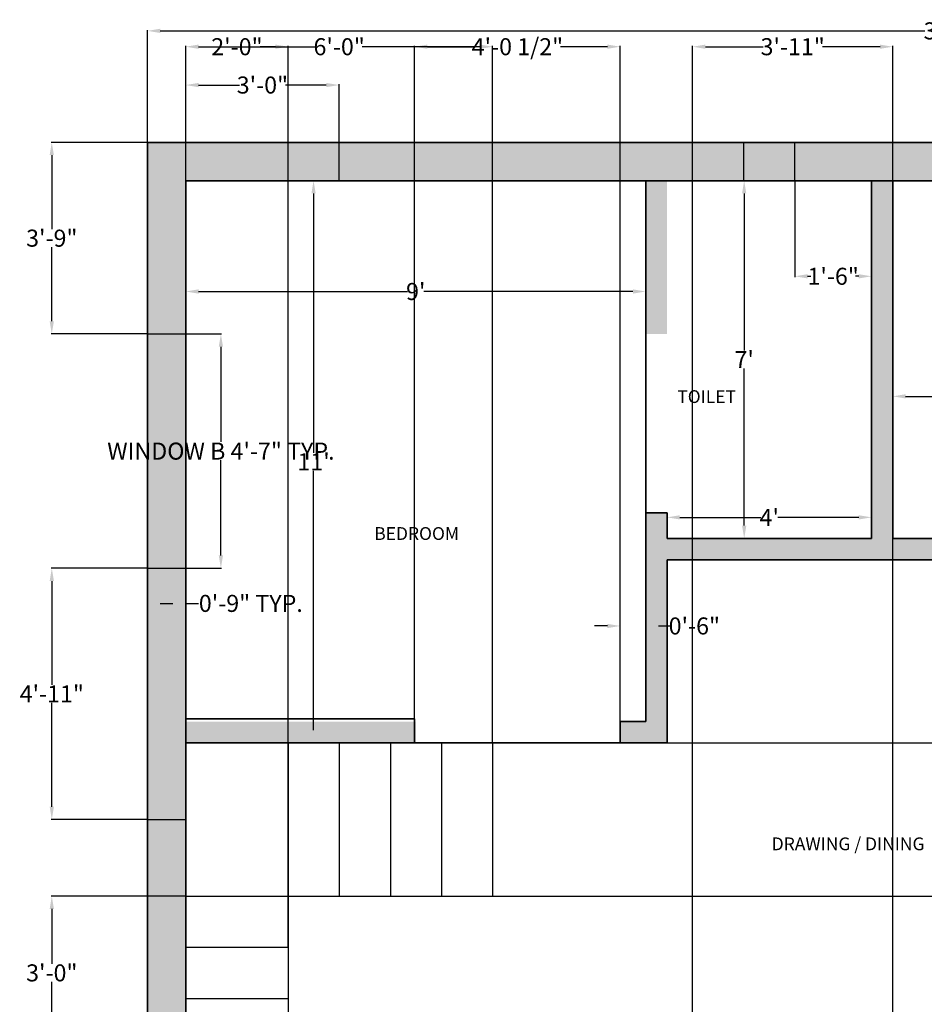
# Model space of a CAD drawing. Units: inches. Extents: x 477 to 929, y 265 to 727.
# Tile 3 of 4: x 477 to 690, y 496 to 727. Entities that reach past the tile are written whole.
import ezdxf

# ---------------------------------------------------------------- set-up
doc = ezdxf.new("R2010")
doc.units = ezdxf.units.IN
doc.header["$MEASUREMENT"] = 0
doc.layers.add('A-ANNO-DIMS', color=215, linetype='Continuous', lineweight=18, true_color=0xa953a0)
doc.layers.add('A-WALL-PATT', color=244, linetype='Continuous', lineweight=13, true_color=0x991b1e)
for name, color, linetype, lineweight in [('A-AREA-IDEN', 3, 'Continuous', 25), ('A-FLOR-STRS', 7, 'Continuous', 25), ('A-GLAZ', 4, 'Continuous', 25), ('A-GLAZ-PATT', 7, 'Continuous', 13), ('A-WALL', 7, 'Continuous', 35)]:
    doc.layers.add(name, color=color, linetype=linetype, lineweight=lineweight)
doc.styles.get("Standard").update_dxf_attribs({"font": 'arial.ttf'})
doc.dimstyles.get("Standard").update_dxf_attribs({"dimtxt": 4, "dimasz": 3, "dimexe": 0.18, "dimexo": 0.0625, "dimgap": 0.09, "dimtad": 0, "dimtih": 1, "dimtoh": 1, "dimdec": 0, "dimzin": 0, "dimdsep": 46, "dimlunit": 3, "dimtxsty": 'Standard', "dimcen": 0, "dimadec": 0, "dimazin": 0, "dimtfac": 1, "dimtdec": 0, "dimtofl": 0, "dimtmove": 0, "dimatfit": 3, "dimfxl": 1, "dimtolj": 1, "dimtzin": 0, "dimarcsym": 1})

# ---------------------------------------------------------------- blocks, each defined once
blk = doc.blocks.new('*D11')
at = {"layer": 'A-ANNO-DIMS', "color": 0, "lineweight": -2, "transparency": 16777216}
for p, q in [((682.33, 605.27), (682.33, 638.75)), ((685.33, 638.57), (704.32, 638.57)), ((727.33, 638.57), (708.34, 638.57)), ((730.33, 605.27), (730.33, 638.75))]:
    blk.add_line(p, q, dxfattribs=at)
at = {"layer": 'A-ANNO-DIMS', "color": 0, "transparency": 16777216}
for points in [[(685.33, 639.07), (685.33, 638.07), (682.33, 638.57)], [(727.33, 639.07), (727.33, 638.07), (730.33, 638.57)]]:
    blk.add_solid(points, dxfattribs=at)
at = {"layer": 'Defpoints', "color": 0, "transparency": 16777216}
for p in [(730.33, 638.57), (682.33, 605.21), (730.33, 605.21)]:
    blk.add_point(p, dxfattribs=at)
at = {"layer": 'A-ANNO-DIMS', "color": 0, "transparency": 16777216, "insert": (706.33, 638.57), "char_height": 4, "attachment_point": 5}
blk.add_mtext("\\A1;4'", dxfattribs=at)
blk = doc.blocks.new('*D13')
at = {"layer": 'A-ANNO-DIMS', "color": 0, "lineweight": -2, "transparency": 16777216}
for p, q in [((629.33, 611.14), (629.33, 609.98)), ((677.33, 611.14), (677.33, 609.98)), ((632.33, 610.16), (651.32, 610.16)), ((674.33, 610.16), (655.34, 610.16))]:
    blk.add_line(p, q, dxfattribs=at)
at = {"layer": 'A-ANNO-DIMS', "color": 0, "transparency": 16777216}
for points in [[(632.33, 610.66), (632.33, 609.66), (629.33, 610.16)], [(674.33, 610.66), (674.33, 609.66), (677.33, 610.16)]]:
    blk.add_solid(points, dxfattribs=at)
at = {"layer": 'Defpoints', "color": 0, "transparency": 16777216}
for p in [(629.33, 611.21), (677.33, 611.21), (677.33, 610.16)]:
    blk.add_point(p, dxfattribs=at)
at = {"layer": 'A-ANNO-DIMS', "color": 0, "transparency": 16777216, "insert": (653.33, 610.16), "char_height": 4, "attachment_point": 5}
blk.add_mtext("\\A1;4'", dxfattribs=at)
blk = doc.blocks.new('*D14')
at = {"layer": 'A-ANNO-DIMS', "color": 0, "lineweight": -2, "transparency": 16777216}
for p, q in [((653.07, 689.21), (647.26, 689.21)), ((647.44, 686.21), (647.44, 649.3)), ((647.44, 608.21), (647.44, 645.12)), ((653.27, 605.21), (647.26, 605.21))]:
    blk.add_line(p, q, dxfattribs=at)
at = {"layer": 'A-ANNO-DIMS', "color": 0, "transparency": 16777216}
for points in [[(646.94, 686.21), (647.94, 686.21), (647.44, 689.21)], [(646.94, 608.21), (647.94, 608.21), (647.44, 605.21)]]:
    blk.add_solid(points, dxfattribs=at)
at = {"layer": 'Defpoints', "color": 0, "transparency": 16777216}
for p in [(653.13, 689.21), (647.44, 605.21), (653.33, 605.21)]:
    blk.add_point(p, dxfattribs=at)
at = {"layer": 'A-ANNO-DIMS', "color": 0, "transparency": 16777216, "insert": (647.44, 647.21), "char_height": 4, "attachment_point": 5}
blk.add_mtext("\\A1;7'", dxfattribs=at)
blk = doc.blocks.new('*D15')
at = {"layer": 'A-ANNO-DIMS', "color": 0, "lineweight": -2, "transparency": 16777216}
for p, q in [((570.81, 689.21), (546.16, 689.21)), ((546.34, 686.21), (546.34, 625.3)), ((546.34, 560.21), (546.34, 621.11)), ((572.77, 557.21), (546.16, 557.21))]:
    blk.add_line(p, q, dxfattribs=at)
at = {"layer": 'A-ANNO-DIMS', "color": 0, "transparency": 16777216}
for points in [[(545.84, 686.21), (546.84, 686.21), (546.34, 689.21)], [(545.84, 560.21), (546.84, 560.21), (546.34, 557.21)]]:
    blk.add_solid(points, dxfattribs=at)
at = {"layer": 'Defpoints', "color": 0, "transparency": 16777216}
for p in [(570.87, 689.21), (546.34, 557.21), (572.83, 557.21)]:
    blk.add_point(p, dxfattribs=at)
at = {"layer": 'A-ANNO-DIMS', "color": 0, "transparency": 16777216, "insert": (546.34, 623.21), "char_height": 4, "attachment_point": 5}
blk.add_mtext("\\A1;11'", dxfattribs=at)
blk = doc.blocks.new('*D16')
at = {"layer": 'A-ANNO-DIMS', "color": 0, "lineweight": -2, "transparency": 16777216}
for p, q in [((516.33, 661.56), (516.33, 663.37)), ((519.33, 663.19), (568.4, 663.19)), ((621.33, 663.19), (572.26, 663.19)), ((624.33, 661.56), (624.33, 663.37))]:
    blk.add_line(p, q, dxfattribs=at)
at = {"layer": 'A-ANNO-DIMS', "color": 0, "transparency": 16777216}
for points in [[(519.33, 663.69), (519.33, 662.69), (516.33, 663.19)], [(621.33, 663.69), (621.33, 662.69), (624.33, 663.19)]]:
    blk.add_solid(points, dxfattribs=at)
at = {"layer": 'Defpoints', "color": 0, "transparency": 16777216}
for p in [(516.33, 661.5), (624.33, 663.19), (624.33, 661.5)]:
    blk.add_point(p, dxfattribs=at)
at = {"layer": 'A-ANNO-DIMS', "color": 0, "transparency": 16777216, "insert": (570.33, 663.19), "char_height": 4, "attachment_point": 5}
blk.add_mtext("\\A1;9'", dxfattribs=at)
blk = doc.blocks.new('*D18')
at = {"layer": 'A-ANNO-DIMS', "color": 0, "lineweight": -2, "transparency": 16777216}
for p, q in [((507.33, 698.27), (507.33, 724.56)), ((510.33, 724.38), (689.88, 724.38)), ((876.4, 724.38), (696.85, 724.38)), ((879.4, 698.27), (879.4, 724.56))]:
    blk.add_line(p, q, dxfattribs=at)
at = {"layer": 'A-ANNO-DIMS', "color": 0, "transparency": 16777216}
for points in [[(510.33, 724.88), (510.33, 723.88), (507.33, 724.38)], [(876.4, 724.88), (876.4, 723.88), (879.4, 724.38)]]:
    blk.add_solid(points, dxfattribs=at)
at = {"layer": 'Defpoints', "color": 0, "transparency": 16777216}
for p in [(879.4, 724.38), (507.33, 698.21), (879.4, 698.21)]:
    blk.add_point(p, dxfattribs=at)
at = {"layer": 'A-ANNO-DIMS', "color": 0, "transparency": 16777216, "insert": (693.36, 724.38), "char_height": 4, "attachment_point": 5}
blk.add_mtext("\\A1;31'", dxfattribs=at)
blk = doc.blocks.new('WIN-JAMBS-36IN')
for p, q in [((9, 36), (0, 36)), ((9, 0), (0, 0))]:
    blk.add_line(p, q)
blk = doc.blocks.new('WIN-JAMBS-55IN')
for p, q in [((0, 55), (9, 55)), ((0, 0), (9, 0))]:
    blk.add_line(p, q)
blk = doc.blocks.new('WIN-JAMBS-12IN')
for p, q in [((0, 0), (0, 9)), ((12, 0), (12, 9))]:
    blk.add_line(p, q)
blk = doc.blocks.new('*D25')
at = {"layer": 'A-ANNO-DIMS', "color": 0, "lineweight": -2, "transparency": 16777216}
for p, q in [((516.4, 653.21), (524.76, 653.21)), ((524.58, 650.21), (524.58, 627.86)), ((524.58, 601.21), (524.58, 623.55)), ((516.4, 598.21), (524.76, 598.21))]:
    blk.add_line(p, q, dxfattribs=at)
at = {"layer": 'A-ANNO-DIMS', "color": 0, "transparency": 16777216}
for points in [[(524.08, 650.21), (525.08, 650.21), (524.58, 653.21)], [(524.08, 601.21), (525.08, 601.21), (524.58, 598.21)]]:
    blk.add_solid(points, dxfattribs=at)
at = {"layer": 'Defpoints', "color": 0, "transparency": 16777216}
for p in [(516.33, 653.21), (524.58, 653.21), (516.33, 598.21)]:
    blk.add_point(p, dxfattribs=at)
at = {"layer": 'A-ANNO-DIMS', "color": 0, "transparency": 16777216, "insert": (524.58, 625.71), "char_height": 4, "attachment_point": 5}
blk.add_mtext('\\A1;WINDOW B 4\'-7" TYP.', dxfattribs=at)
blk = doc.blocks.new('*D26')
at = {"layer": 'A-ANNO-DIMS', "color": 0, "lineweight": -2, "transparency": 16777216}
for p, q in [((507.33, 598.14), (507.33, 589.78)), ((516.33, 598.14), (516.33, 589.78)), ((510.33, 589.96), (513.33, 589.96)), ((516.33, 589.96), (519.33, 589.96))]:
    blk.add_line(p, q, dxfattribs=at)
at = {"layer": 'A-ANNO-DIMS', "color": 0, "transparency": 16777216}
for points in [[(510.33, 590.46), (510.33, 589.46), (507.33, 589.96)], [(513.33, 590.46), (513.33, 589.46), (516.33, 589.96)]]:
    blk.add_solid(points, dxfattribs=at)
at = {"layer": 'Defpoints', "color": 0, "transparency": 16777216}
for p in [(507.33, 598.21), (516.33, 598.21), (516.33, 589.96)]:
    blk.add_point(p, dxfattribs=at)
at = {"layer": 'A-ANNO-DIMS', "color": 0, "transparency": 16777216, "insert": (531.61, 589.96), "char_height": 4, "attachment_point": 5}
blk.add_mtext('\\A1;0\'-9" TYP.', dxfattribs=at)
blk = doc.blocks.new('*D30')
at = {"layer": 'A-ANNO-DIMS', "color": 0, "lineweight": -2, "transparency": 16777216}
for p, q in [((588.43, 557.21), (901.96, 557.21)), ((901.78, 554.21), (901.78, 541.34)), ((901.78, 524.21), (901.78, 537.07)), ((588.43, 521.21), (901.96, 521.21))]:
    blk.add_line(p, q, dxfattribs=at)
at = {"layer": 'A-ANNO-DIMS', "color": 0, "transparency": 16777216}
for points in [[(901.28, 554.21), (902.28, 554.21), (901.78, 557.21)], [(901.28, 524.21), (902.28, 524.21), (901.78, 521.21)]]:
    blk.add_solid(points, dxfattribs=at)
at = {"layer": 'Defpoints', "color": 0, "transparency": 16777216}
for p in [(588.37, 557.21), (901.78, 557.21), (588.37, 521.21)]:
    blk.add_point(p, dxfattribs=at)
at = {"layer": 'A-ANNO-DIMS', "color": 0, "transparency": 16777216, "insert": (901.78, 539.21), "char_height": 4, "attachment_point": 5}
blk.add_mtext('\\A1;3\'-0"', dxfattribs=at)
blk = doc.blocks.new('*D32')
at = {"layer": 'A-ANNO-DIMS', "color": 0, "lineweight": -2, "transparency": 16777216}
for p, q in [((516.33, 509.27), (516.33, 720.84)), ((519.33, 720.66), (522.91, 720.66)), ((537.37, 720.66), (533.79, 720.66)), ((540.37, 509.27), (540.37, 720.84))]:
    blk.add_line(p, q, dxfattribs=at)
at = {"layer": 'A-ANNO-DIMS', "color": 0, "transparency": 16777216}
for points in [[(519.33, 721.16), (519.33, 720.16), (516.33, 720.66)], [(537.37, 721.16), (537.37, 720.16), (540.37, 720.66)]]:
    blk.add_solid(points, dxfattribs=at)
at = {"layer": 'Defpoints', "color": 0, "transparency": 16777216}
for p in [(540.37, 720.66), (516.33, 509.21), (540.37, 509.21)]:
    blk.add_point(p, dxfattribs=at)
at = {"layer": 'A-ANNO-DIMS', "color": 0, "transparency": 16777216, "insert": (528.35, 720.66), "char_height": 4, "attachment_point": 5}
blk.add_mtext('\\A1;2\'-0"', dxfattribs=at)
blk = doc.blocks.new('*D33')
at = {"layer": 'A-ANNO-DIMS', "color": 0, "lineweight": -2, "transparency": 16777216}
for p, q in [((516.33, 557.27), (516.33, 720.84)), ((519.33, 720.66), (546.93, 720.66)), ((585.37, 720.66), (557.77, 720.66)), ((588.37, 557.27), (588.37, 720.84))]:
    blk.add_line(p, q, dxfattribs=at)
at = {"layer": 'A-ANNO-DIMS', "color": 0, "transparency": 16777216}
for points in [[(519.33, 721.16), (519.33, 720.16), (516.33, 720.66)], [(585.37, 721.16), (585.37, 720.16), (588.37, 720.66)]]:
    blk.add_solid(points, dxfattribs=at)
at = {"layer": 'Defpoints', "color": 0, "transparency": 16777216}
for p in [(588.37, 720.66), (516.33, 557.21), (588.37, 557.21)]:
    blk.add_point(p, dxfattribs=at)
at = {"layer": 'A-ANNO-DIMS', "color": 0, "transparency": 16777216, "insert": (552.35, 720.66), "char_height": 4, "attachment_point": 5}
blk.add_mtext('\\A1;6\'-0"', dxfattribs=at)
blk = doc.blocks.new('*D35')
at = {"layer": 'A-ANNO-DIMS', "color": 0, "lineweight": -2, "transparency": 16777216}
for p, q in [((516.27, 521.21), (484.7, 521.21)), ((484.88, 518.21), (484.88, 505.34)), ((484.88, 488.21), (484.88, 501.07)), ((516.27, 485.21), (484.7, 485.21))]:
    blk.add_line(p, q, dxfattribs=at)
at = {"layer": 'A-ANNO-DIMS', "color": 0, "transparency": 16777216}
for points in [[(484.38, 518.21), (485.38, 518.21), (484.88, 521.21)], [(484.38, 488.21), (485.38, 488.21), (484.88, 485.21)]]:
    blk.add_solid(points, dxfattribs=at)
at = {"layer": 'Defpoints', "color": 0, "transparency": 16777216}
for p in [(484.88, 521.21), (516.33, 521.21), (516.33, 485.21)]:
    blk.add_point(p, dxfattribs=at)
at = {"layer": 'A-ANNO-DIMS', "color": 0, "transparency": 16777216, "insert": (484.88, 503.21), "char_height": 4, "attachment_point": 5}
blk.add_mtext('\\A1;3\'-0"', dxfattribs=at)
blk = doc.blocks.new('*D40')
at = {"layer": 'A-ANNO-DIMS', "color": 0, "lineweight": -2, "transparency": 16777216}
for p, q in [((516.33, 689.27), (516.33, 711.84)), ((519.33, 711.66), (528.93, 711.66)), ((549.33, 711.66), (539.74, 711.66)), ((552.33, 689.27), (552.33, 711.84))]:
    blk.add_line(p, q, dxfattribs=at)
at = {"layer": 'A-ANNO-DIMS', "color": 0, "transparency": 16777216}
for points in [[(519.33, 712.16), (519.33, 711.16), (516.33, 711.66)], [(549.33, 712.16), (549.33, 711.16), (552.33, 711.66)]]:
    blk.add_solid(points, dxfattribs=at)
at = {"layer": 'Defpoints', "color": 0, "transparency": 16777216}
for p in [(552.33, 711.66), (516.33, 689.21), (552.33, 689.21)]:
    blk.add_point(p, dxfattribs=at)
at = {"layer": 'A-ANNO-DIMS', "color": 0, "transparency": 16777216, "insert": (534.33, 711.66), "char_height": 4, "attachment_point": 5}
blk.add_mtext('\\A1;3\'-0"', dxfattribs=at)
blk = doc.blocks.new('*D41')
at = {"layer": 'A-ANNO-DIMS', "color": 0, "lineweight": -2, "transparency": 16777216}
for p, q in [((659.33, 689.14), (659.33, 666.58)), ((677.33, 689.14), (677.33, 666.58)), ((662.33, 666.76), (663.12, 666.76)), ((674.33, 666.76), (673.55, 666.76))]:
    blk.add_line(p, q, dxfattribs=at)
at = {"layer": 'A-ANNO-DIMS', "color": 0, "transparency": 16777216}
for points in [[(662.33, 667.26), (662.33, 666.26), (659.33, 666.76)], [(674.33, 667.26), (674.33, 666.26), (677.33, 666.76)]]:
    blk.add_solid(points, dxfattribs=at)
at = {"layer": 'Defpoints', "color": 0, "transparency": 16777216}
for p in [(659.33, 689.21), (677.33, 689.21), (659.33, 666.76)]:
    blk.add_point(p, dxfattribs=at)
at = {"layer": 'A-ANNO-DIMS', "color": 0, "transparency": 16777216, "insert": (668.33, 666.76), "char_height": 4, "attachment_point": 5}
blk.add_mtext('\\A1;1\'-6"', dxfattribs=at)
blk = doc.blocks.new('*D45')
at = {"layer": 'A-ANNO-DIMS', "color": 0, "lineweight": -2, "transparency": 16777216}
for p, q in [((507.27, 698.21), (484.7, 698.21)), ((484.88, 695.21), (484.88, 677.84)), ((484.88, 656.21), (484.88, 673.57)), ((507.27, 653.21), (484.7, 653.21))]:
    blk.add_line(p, q, dxfattribs=at)
at = {"layer": 'A-ANNO-DIMS', "color": 0, "transparency": 16777216}
for points in [[(484.38, 695.21), (485.38, 695.21), (484.88, 698.21)], [(484.38, 656.21), (485.38, 656.21), (484.88, 653.21)]]:
    blk.add_solid(points, dxfattribs=at)
at = {"layer": 'Defpoints', "color": 0, "transparency": 16777216}
for p in [(484.88, 698.21), (507.33, 698.21), (507.33, 653.21)]:
    blk.add_point(p, dxfattribs=at)
at = {"layer": 'A-ANNO-DIMS', "color": 0, "transparency": 16777216, "insert": (484.88, 675.71), "char_height": 4, "attachment_point": 5}
blk.add_mtext('\\A1;3\'-9"', dxfattribs=at)
blk = doc.blocks.new('*D46')
at = {"layer": 'A-ANNO-DIMS', "color": 0, "lineweight": -2, "transparency": 16777216}
for p, q in [((507.27, 598.21), (484.7, 598.21)), ((484.88, 595.21), (484.88, 570.8)), ((484.88, 542.21), (484.88, 566.61)), ((507.27, 539.21), (484.7, 539.21))]:
    blk.add_line(p, q, dxfattribs=at)
at = {"layer": 'A-ANNO-DIMS', "color": 0, "transparency": 16777216}
for points in [[(484.38, 595.21), (485.38, 595.21), (484.88, 598.21)], [(484.38, 542.21), (485.38, 542.21), (484.88, 539.21)]]:
    blk.add_solid(points, dxfattribs=at)
at = {"layer": 'Defpoints', "color": 0, "transparency": 16777216}
for p in [(484.88, 598.21), (507.33, 598.21), (507.33, 539.21)]:
    blk.add_point(p, dxfattribs=at)
at = {"layer": 'A-ANNO-DIMS', "color": 0, "transparency": 16777216, "insert": (484.88, 568.71), "char_height": 4, "attachment_point": 5}
blk.add_mtext('\\A1;4\'-11"', dxfattribs=at)
blk = doc.blocks.new('*D57')
at = {"layer": 'A-ANNO-DIMS', "color": 0, "lineweight": -2, "transparency": 16777216}
for p, q in [((635.33, 400.27), (635.33, 720.84)), ((638.33, 720.66), (651.87, 720.66)), ((679.33, 720.66), (665.79, 720.66)), ((682.33, 400.27), (682.33, 720.84))]:
    blk.add_line(p, q, dxfattribs=at)
at = {"layer": 'A-ANNO-DIMS', "color": 0, "transparency": 16777216}
for points in [[(638.33, 721.16), (638.33, 720.16), (635.33, 720.66)], [(679.33, 721.16), (679.33, 720.16), (682.33, 720.66)]]:
    blk.add_solid(points, dxfattribs=at)
at = {"layer": 'Defpoints', "color": 0, "transparency": 16777216}
for p in [(682.33, 720.66), (635.33, 400.21), (682.33, 400.21)]:
    blk.add_point(p, dxfattribs=at)
at = {"layer": 'A-ANNO-DIMS', "color": 0, "transparency": 16777216, "insert": (658.83, 720.66), "char_height": 4, "attachment_point": 5}
blk.add_mtext('\\A1;3\'-11"', dxfattribs=at)
blk = doc.blocks.new('*D61')
at = {"layer": 'A-ANNO-DIMS', "color": 0, "lineweight": -2, "transparency": 16777216}
for p, q in [((570.07, 562.88), (570.07, 720.84)), ((573.07, 720.66), (584.05, 720.66)), ((615.33, 720.66), (604.35, 720.66)), ((618.33, 562.27), (618.33, 720.84))]:
    blk.add_line(p, q, dxfattribs=at)
at = {"layer": 'A-ANNO-DIMS', "color": 0, "transparency": 16777216}
for points in [[(573.07, 721.16), (573.07, 720.16), (570.07, 720.66)], [(615.33, 721.16), (615.33, 720.16), (618.33, 720.66)]]:
    blk.add_solid(points, dxfattribs=at)
at = {"layer": 'Defpoints', "color": 0, "transparency": 16777216}
for p in [(570.07, 720.66), (570.07, 562.82), (618.33, 562.21)]:
    blk.add_point(p, dxfattribs=at)
at = {"layer": 'A-ANNO-DIMS', "color": 0, "transparency": 16777216, "insert": (594.2, 720.66), "char_height": 4, "attachment_point": 5}
blk.add_mtext('\\A1;4\'-0 1/2"', dxfattribs=at)
blk = doc.blocks.new('*D68')
at = {"layer": 'A-ANNO-DIMS', "color": 0, "lineweight": -2, "transparency": 16777216}
for p, q in [((615.33, 584.66), (612.33, 584.66)), ((618.33, 562.27), (618.33, 584.84)), ((624.33, 562.27), (624.33, 584.84)), ((627.33, 584.66), (630.33, 584.66))]:
    blk.add_line(p, q, dxfattribs=at)
at = {"layer": 'A-ANNO-DIMS', "color": 0, "transparency": 16777216}
for points in [[(615.33, 585.16), (615.33, 584.16), (618.33, 584.66)], [(627.33, 585.16), (627.33, 584.16), (624.33, 584.66)]]:
    blk.add_solid(points, dxfattribs=at)
at = {"layer": 'Defpoints', "color": 0, "transparency": 16777216}
for p in [(624.33, 584.66), (618.33, 562.21), (624.33, 562.21)]:
    blk.add_point(p, dxfattribs=at)
at = {"layer": 'A-ANNO-DIMS', "color": 0, "transparency": 16777216, "insert": (635.74, 584.66), "char_height": 4, "attachment_point": 5}
blk.add_mtext('\\A1;0\'-6"', dxfattribs=at)

msp = doc.modelspace()

# ---------------------------------------------------------------- hatches: boundary and pattern name
at = {"layer": 'A-GLAZ-PATT'}
h = msp.add_hatch(color=256, dxfattribs=at)
h.dxf.hatch_style = 1
h.paths.add_polyline_path([(588.33, 698.21), (552.33, 698.21), (552.33, 689.21), (588.33, 689.21)])
h.paths.add_polyline_path([(659.33, 698.21), (647.33, 698.21), (647.33, 689.21), (659.33, 689.21)])
h.paths.add_polyline_path([(712.33, 698.21), (700.33, 698.21), (700.33, 689.21), (712.33, 689.21)])
h.paths.add_polyline_path([(834.33, 698.21), (771.33, 698.21), (771.33, 689.21), (834.33, 689.21)])
h.paths.add_polyline_path([(879.33, 653.21), (870.33, 653.21), (870.33, 598.21), (879.33, 598.21)])
h.paths.add_polyline_path([(879.33, 521.21), (870.33, 521.21), (870.33, 484.21), (879.33, 484.21)])
h.paths.add_polyline_path([(879.33, 407.21), (870.33, 407.21), (870.33, 371.21), (879.33, 371.21)])
h.paths.add_polyline_path([(834.33, 335.21), (766.33, 335.21), (766.33, 326.21), (834.33, 326.21)])
h.paths.add_polyline_path([(588.33, 335.21), (552.33, 335.21), (552.33, 326.21), (588.33, 326.21)])
h.paths.add_polyline_path([(516.33, 430.21), (507.33, 430.21), (507.33, 371.21), (516.33, 371.21)])
h.paths.add_polyline_path([(516.33, 539.21), (507.33, 539.21), (507.33, 466.21), (516.33, 466.21)])
h.paths.add_polyline_path([(516.33, 653.21), (507.33, 653.21), (507.33, 598.21), (516.33, 598.21)])
at = {"layer": 'A-WALL-PATT'}
h = msp.add_hatch(color=256, dxfattribs=at)
h.dxf.hatch_style = 1
h.paths.add_polyline_path([(516.33, 598.21), (507.33, 598.21), (507.33, 539.21), (516.33, 539.21), (516.33, 557.21), (570.33, 557.21), (570.33, 562.21), (516.33, 562.21)])
h.paths.add_polyline_path([(552.33, 698.21), (507.33, 698.21), (507.33, 653.21), (516.33, 653.21), (516.33, 689.21), (552.33, 689.21)])
h.paths.add_polyline_path([(647.33, 698.21), (588.33, 698.21), (588.33, 689.21), (647.33, 689.21)])
h.paths.add_polyline_path([(700.33, 698.21), (659.33, 698.21), (659.33, 689.21), (700.33, 689.21)])
h.paths.add_polyline_path([(771.33, 698.21), (712.33, 698.21), (712.33, 689.21), (771.33, 689.21)])
h.paths.add_polyline_path([(879.33, 698.21), (834.33, 698.21), (834.33, 689.21), (870.33, 689.21), (870.33, 653.21), (879.33, 653.21)])
h.paths.add_polyline_path([(879.33, 598.21), (870.33, 598.21), (870.33, 562.21), (735.33, 562.21), (735.33, 568.21), (730.33, 568.21), (730.33, 557.21), (793.33, 557.21), (793.33, 551.21), (798.33, 551.21), (798.33, 557.21), (870.33, 557.21), (870.33, 521.21), (879.33, 521.21)])
h.paths.add_polyline_path([(879.33, 484.21), (870.33, 484.21), (870.33, 448.21), (798.33, 448.21), (798.33, 495.83), (793.33, 495.83), (793.33, 448.21), (788.33, 448.21), (788.33, 443.21), (870.33, 443.21), (870.33, 407.21), (879.33, 407.21)])
h.paths.add_polyline_path([(735.33, 443.21), (740.33, 443.21), (740.33, 448.21), (730.33, 448.21), (730.33, 400.21), (682.33, 400.21), (682.33, 395.21), (730.33, 395.21), (730.33, 326.21), (766.33, 326.21), (766.33, 335.21), (735.33, 335.21)])
h.paths.add_polyline_path([(879.33, 371.21), (870.33, 371.21), (870.33, 335.21), (834.33, 335.21), (834.33, 326.21), (879.33, 326.21)])
h.paths.add_polyline_path([(516.33, 466.21), (507.33, 466.21), (507.33, 430.21), (516.33, 430.21), (516.33, 443.21), (624.33, 443.21), (624.33, 437.21), (629.33, 437.21), (629.33, 448.21), (516.33, 448.21)])
h.paths.add_polyline_path([(629.33, 600.21), (700.33, 600.21), (700.33, 605.21), (682.33, 605.21), (682.33, 689.21), (677.33, 689.21), (677.33, 605.21), (629.33, 605.21), (629.33, 611.21), (624.33, 611.21), (624.33, 562.21), (618.33, 562.21), (618.33, 557.21), (629.33, 557.21)])
h.paths.add_polyline_path([(629.33, 689.21), (624.33, 689.21), (624.33, 653.21), (629.33, 653.21)], flags=17)

# ---------------------------------------------------------------- linework, layer by layer
at = {"layer": 'A-FLOR-STRS'}
for p, q in [((540.37, 557.21), (540.37, 448.21)), ((552.37, 557.21), (552.37, 521.21)), ((564.37, 557.21), (564.37, 521.21)), ((576.37, 557.21), (576.37, 521.21)), ((588.37, 557.21), (588.37, 521.21)), ((516.33, 521.21), (588.37, 521.21)), ((516.33, 509.21), (540.37, 509.21)), ((516.33, 497.21), (540.37, 497.21))]:
    msp.add_line(p, q, dxfattribs=at)
at = {"layer": 'A-GLAZ'}
msp.add_line((507.33, 539.21), (516.33, 539.21), dxfattribs=at)
at = {"layer": 'A-WALL'}
for p, q in [((507.33, 698.21), (879.33, 698.21)), ((507.33, 326.21), (507.33, 698.21)), ((879.33, 698.21), (507.33, 698.21)), ((507.33, 698.21), (507.33, 326.21)), ((516.33, 689.21), (870.33, 689.21)), ((516.33, 557.21), (516.33, 689.21)), ((516.33, 689.21), (870.33, 689.21)), ((624.33, 562.21), (624.33, 689.21)), ((677.33, 605.21), (677.33, 689.21)), ((682.33, 605.21), (682.33, 689.21)), ((624.33, 611.21), (629.33, 611.21)), ((629.33, 605.21), (629.33, 611.21)), ((629.33, 605.21), (677.33, 605.21)), ((682.33, 605.21), (700.33, 605.21)), ((629.33, 600.21), (730.33, 600.21)), ((629.33, 557.21), (629.33, 600.21)), ((516.33, 562.82), (570.07, 562.82)), ((570.07, 562.82), (570.07, 557.21)), ((618.33, 557.21), (618.33, 562.21)), ((618.33, 562.21), (624.33, 562.21)), ((618.33, 562.21), (624.33, 562.21)), ((516.33, 557.21), (629.33, 557.21)), ((516.33, 557.21), (629.33, 557.21)), ((516.33, 448.21), (516.33, 557.21))]:
    msp.add_line(p, q, dxfattribs=at)

# ---------------------------------------------------------------- block references
at = {"layer": 'A-GLAZ', "rotation": 270.0000000000003}
msp.add_blockref('WIN-JAMBS-36IN', (552.33, 698.21), dxfattribs=at)
at = {"layer": 'A-GLAZ'}
for name, p in [('WIN-JAMBS-12IN', (647.33, 689.21)), ('WIN-JAMBS-55IN', (507.33, 598.21))]:
    msp.add_blockref(name, p, dxfattribs=at)

# ---------------------------------------------------------------- texts
at = {"layer": 'A-AREA-IDEN'}
msp.add_text('TOILET', height=3, dxfattribs=at).set_placement((631.74, 637.01))
at = {"layer": 'A-AREA-IDEN', "char_height": 3, "attachment_point": 1}
for s, width, insert in [('BEDROOM', 102.2555, (560.59, 607.86)), ('DRAWING / DINING', 101.5163, (653.91, 535))]:
    msp.add_mtext_dynamic_manual_height_columns(s, width=width, gutter_width=1, heights=[0], dxfattribs=dict(at, insert=insert))

# ---------------------------------------------------------------- dimensions: what is measured, and where the dimension line sits
at = {"layer": 'A-ANNO-DIMS'}
for base, p1, p2, override, picture, middle in [((879.4, 724.38), (507.33, 698.21), (879.4, 698.21), {"dimclrd": 0, "dimclre": 0, "dimclrt": 0}, '*D18', (693.36, 724.38)), ((570.07, 720.66), (618.33, 562.21), (570.07, 562.82), {"dimdec": 1, "dimlfac": 1, "dimrnd": 0, "dimzin": 1, "dimdsep": 46, "dimlunit": 4, "dimfrac": 2}, '*D61', (594.2, 720.66)), ((540.37, 720.66), (516.33, 509.21), (540.37, 509.21), {"dimdec": 1, "dimlfac": 1, "dimrnd": 0, "dimzin": 1, "dimdsep": 46, "dimlunit": 4, "dimfrac": 2}, '*D32', (528.35, 720.66)), ((588.37, 720.66), (516.33, 557.21), (588.37, 557.21), {"dimdec": 1, "dimlfac": 1, "dimrnd": 0, "dimzin": 1, "dimdsep": 46, "dimlunit": 4, "dimfrac": 2}, '*D33', (552.35, 720.66)), ((682.33, 720.66), (635.33, 400.21), (682.33, 400.21), {"dimdec": 1, "dimlfac": 1, "dimrnd": 0, "dimzin": 1, "dimdsep": 46, "dimlunit": 4, "dimfrac": 2}, '*D57', (658.83, 720.66)), ((552.33, 711.66), (516.33, 689.21), (552.33, 689.21), {"dimdec": 1, "dimlfac": 1, "dimrnd": 0, "dimzin": 1, "dimdsep": 46, "dimlunit": 4, "dimfrac": 2}, '*D40', (534.33, 711.66)), ((624.33, 663.19), (516.33, 661.5), (624.33, 661.5), {"dimclrd": 0, "dimclre": 0, "dimclrt": 0}, '*D16', (570.33, 663.19)), ((730.33, 638.57), (682.33, 605.21), (730.33, 605.21), {"dimclrd": 0, "dimclre": 0, "dimclrt": 0}, '*D11', (706.33, 638.57)), ((677.33, 610.16), (629.33, 611.21), (677.33, 611.21), {"dimclrd": 0, "dimclre": 0, "dimclrt": 0}, '*D13', (653.33, 610.16)), ((624.33, 584.66), (618.33, 562.21), (624.33, 562.21), {"dimdec": 1, "dimlfac": 1, "dimrnd": 0, "dimzin": 1, "dimdsep": 46, "dimlunit": 4, "dimfrac": 2}, '*D68', (635.74, 584.66))]:
    dim = msp.add_linear_dim(base=base, p1=p1, p2=p2, dimstyle='Standard', override=override, dxfattribs=at)
    dim.commit()
    dim.dimension.update_dxf_attribs({"geometry": picture, "text_midpoint": middle})
for base, p1, p2, angle, override, picture, middle in [((484.88, 698.21), (507.33, 653.21), (507.33, 698.21), 90, {"dimdec": 1, "dimlfac": 1, "dimrnd": 0, "dimzin": 1, "dimdsep": 46, "dimlunit": 4, "dimfrac": 2}, '*D45', (484.88, 675.71)), ((546.34, 557.21), (570.87, 689.21), (572.83, 557.21), 90, {"dimclrd": 0, "dimclre": 0, "dimclrt": 0}, '*D15', (546.34, 623.21)), ((647.44, 605.21), (653.13, 689.21), (653.33, 605.21), 90, {"dimclrd": 0, "dimclre": 0, "dimclrt": 0}, '*D14', (647.44, 647.21)), ((659.33, 666.76), (677.33, 689.21), (659.33, 689.21), 180, {"dimdec": 1, "dimlfac": 1, "dimrnd": 0, "dimzin": 1, "dimdsep": 46, "dimlunit": 4, "dimfrac": 2}, '*D41', (668.33, 666.76)), ((484.88, 598.21), (507.33, 539.21), (507.33, 598.21), 90, {"dimdec": 1, "dimlfac": 1, "dimrnd": 0, "dimzin": 1, "dimdsep": 46, "dimlunit": 4, "dimfrac": 2}, '*D46', (484.88, 568.71)), ((901.78, 557.21), (588.37, 521.21), (588.37, 557.21), 90, {"dimdec": 1, "dimlfac": 1, "dimrnd": 0, "dimzin": 1, "dimdsep": 46, "dimlunit": 4, "dimfrac": 2}, '*D30', (901.78, 539.21)), ((484.88, 521.21), (516.33, 485.21), (516.33, 521.21), 90, {"dimdec": 1, "dimlfac": 1, "dimrnd": 0, "dimzin": 1, "dimdsep": 46, "dimlunit": 4, "dimfrac": 2}, '*D35', (484.88, 503.21))]:
    dim = msp.add_linear_dim(base=base, p1=p1, p2=p2, angle=angle, dimstyle='Standard', override=override, dxfattribs=at)
    dim.commit()
    dim.dimension.update_dxf_attribs({"geometry": picture, "text_midpoint": middle})
dim = msp.add_linear_dim(base=(524.58, 653.21), p1=(516.33, 598.21), p2=(516.33, 653.21), angle=90, text='WINDOW B <> TYP.', dimstyle='Standard', override={"dimdec": 1, "dimlfac": 1, "dimrnd": 0, "dimzin": 1, "dimdsep": 46, "dimlunit": 4, "dimfrac": 2}, dxfattribs=at)
dim.commit()
dim.dimension.update_dxf_attribs({"geometry": '*D25', "text_midpoint": (524.58, 625.71)})
dim = msp.add_linear_dim(base=(516.33, 589.96), p1=(507.33, 598.21), p2=(516.33, 598.21), text='<> TYP.', dimstyle='Standard', override={"dimdec": 1, "dimlfac": 1, "dimrnd": 0, "dimzin": 1, "dimdsep": 46, "dimlunit": 4, "dimfrac": 2}, dxfattribs=at)
dim.commit()
dim.dimension.update_dxf_attribs({"geometry": '*D26', "text_midpoint": (531.61, 589.96)})

doc.saveas('drawing.dxf')
